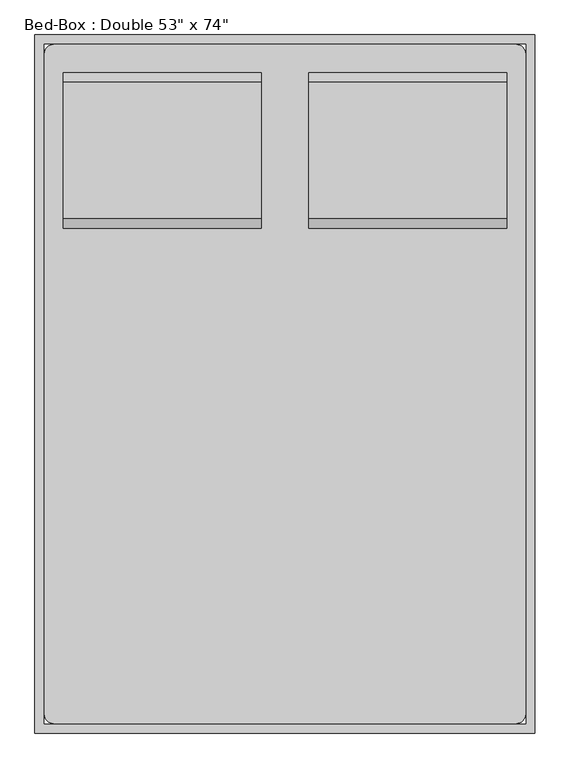
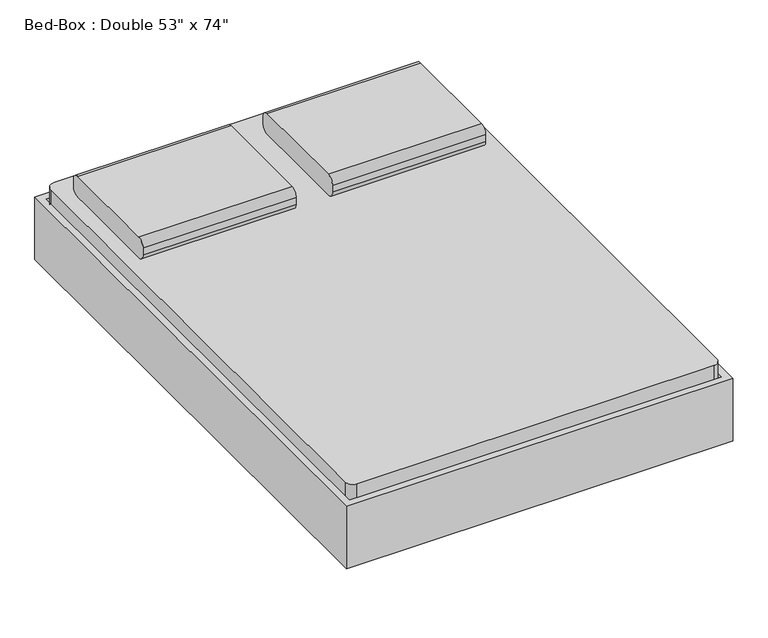
"""IFC4 building model written with IfcOpenShell, lengths in millimetres: furniture geometry."""

from ifc_helpers import new_model, si_unit, point, frame, frame_2d, origin, place, context, project, spatial, polyline, circle_curve, trimmed, segment, composite_curve, outline, extrude, source, transform, mapped, element, save
from ifc_brep_helpers import plane_surface, cylinder_surface, revolved_surface, advanced_brep


def furniture_c8abb964(model_context):
    return source(origin(), model_context, "Body", "SolidModel", [
        extrude(outline(composite_curve([segment(polyline([(578.3704918, 406.4), (210.0704918, 406.4)]), True, "CONTINUOUS"), segment(trimmed(circle_curve(frame_2d((210.0704918, 431.8)), 25.4), [point((210.0704918, 406.4))], [point((184.6704918, 431.8))], False, "CARTESIAN"), True, "CONTINUOUS"), segment(polyline([(184.6704918, 431.8), (184.6704918, 457.2)]), True, "CONTINUOUS"), segment(trimmed(circle_curve(frame_2d((210.0704918, 457.2)), 25.4), [point((184.6704918, 457.2))], [point((210.0704918, 482.6))], False, "CARTESIAN"), True, "CONTINUOUS"), segment(polyline([(210.0704918, 482.6), (578.3704918, 482.6)]), True, "CONTINUOUS"), segment(trimmed(circle_curve(frame_2d((578.3704918, 457.2)), 25.4), [point((578.3704918, 482.6))], [point((603.7704918, 457.2))], False, "CARTESIAN"), True, "CONTINUOUS"), segment(polyline([(603.7704918, 457.2), (603.7704918, 431.8)]), True, "CONTINUOUS"), segment(trimmed(circle_curve(frame_2d((578.3704918, 431.8)), 25.4), [point((603.7704918, 431.8))], [point((578.3704918, 406.4))], False, "CARTESIAN"), True, "CONTINUOUS")], self_intersect=False)), frame((402.652459, 0.0, 0.0), z_axis=(1.0, 0.0, 0.0), x_axis=(0.0, 1.0, 0.0)), (0.0, 0.0, 1.0), 533.4),
        extrude(outline(composite_curve([segment(polyline([(578.3704918, 406.4), (210.0704918, 406.4)]), True, "CONTINUOUS"), segment(trimmed(circle_curve(frame_2d((210.0704918, 431.8)), 25.4), [point((210.0704918, 406.4))], [point((184.6704918, 431.8))], False, "CARTESIAN"), True, "CONTINUOUS"), segment(polyline([(184.6704918, 431.8), (184.6704918, 457.2)]), True, "CONTINUOUS"), segment(trimmed(circle_curve(frame_2d((210.0704918, 457.2)), 25.4), [point((184.6704918, 457.2))], [point((210.0704918, 482.6))], False, "CARTESIAN"), True, "CONTINUOUS"), segment(polyline([(210.0704918, 482.6), (578.3704918, 482.6)]), True, "CONTINUOUS"), segment(trimmed(circle_curve(frame_2d((578.3704918, 457.2)), 25.4), [point((578.3704918, 482.6))], [point((603.7704918, 457.2))], False, "CARTESIAN"), True, "CONTINUOUS"), segment(polyline([(603.7704918, 457.2), (603.7704918, 431.8)]), True, "CONTINUOUS"), segment(trimmed(circle_curve(frame_2d((578.3704918, 431.8)), 25.4), [point((603.7704918, 431.8))], [point((578.3704918, 406.4))], False, "CARTESIAN"), True, "CONTINUOUS")], self_intersect=False)), frame((-257.747541, 0.0, 0.0), z_axis=(1.0, 0.0, 0.0), x_axis=(0.0, 1.0, 0.0)), (0.0, 0.0, 1.0), 533.4),
        advanced_brep(
        [(-308.2231784, 451.3704918, 177.8), (-308.2231784, 375.1704918, 177.8), (-308.2231784, 375.1704918, 196.85), (-308.2231784, 451.3704918, 196.85), (-257.4231784, 451.3704918, 177.8), (-257.4231784, 375.1704918, 177.8), (-245.2869899, 375.1704918, 196.85), (-245.2869899, 451.3704918, 196.85), (-181.3523099, 451.3704918, 14.6654962), (-181.3523099, 375.1704918, 14.6654962), (-164.0871466, 375.1704918, 22.716374), (-164.0871466, 451.3704918, 22.716374), (-158.3320921, 375.1704918, 0.0), (-158.3320921, 451.3704918, 0.0), (-158.3320921, 375.1704918, 19.05), (-158.3320921, 451.3704918, 19.05), (-79.7195862, 451.3704918, 0.0), (-79.7195862, 375.1704918, 0.0), (-79.7195862, 375.1704918, 19.05), (-79.7195862, 451.3704918, 19.05), (-67.0195862, 375.1704918, 3.4029547), (-67.0195862, 451.3704918, 3.4029547), (-76.5445862, 375.1704918, 19.9007387), (-76.5445862, 451.3704918, 19.9007387), (-6.922541, 451.3704918, 38.1), (-6.922541, 375.1704918, 38.1), (-12.0269731, 375.1704918, 57.15), (-12.0269731, 451.3704918, 57.15), (685.5518216, 451.3704918, 38.1), (685.5518216, 375.1704918, 38.1), (690.6562537, 375.1704918, 57.15), (690.6562537, 451.3704918, 57.15), (745.6488669, 451.3704918, 3.4029547), (745.6488669, 375.1704918, 3.4029547), (755.1738669, 375.1704918, 19.9007387), (755.1738669, 451.3704918, 19.9007387), (758.3488669, 375.1704918, 0.0), (758.3488669, 451.3704918, 0.0), (758.3488669, 375.1704918, 19.05), (758.3488669, 451.3704918, 19.05), (836.9613728, 451.3704918, 0.0), (836.9613728, 375.1704918, 0.0), (836.9613728, 375.1704918, 19.05), (836.9613728, 451.3704918, 19.05), (859.9815906, 375.1704918, 14.6654962), (859.9815906, 451.3704918, 14.6654962), (842.7164272, 375.1704918, 22.716374), (842.7164272, 451.3704918, 22.716374), (936.052459, 451.3704918, 177.8), (936.052459, 375.1704918, 177.8), (923.9162705, 375.1704918, 196.85), (923.9162705, 451.3704918, 196.85), (986.852459, 451.3704918, 177.8), (986.852459, 451.3704918, 196.85), (986.852459, 375.1704918, 196.85), (986.852459, 375.1704918, 177.8)],
        [
            (0, 1),
            (1, 2),
            (2, 3),
            (3, 0),
            (0, 4),
            (4, 5),
            (5, 1),
            (5, 6),
            (6, 2),
            (6, 7),
            (7, 3),
            (7, 4),
            (4, 8),
            (8, 9),
            (9, 5),
            (9, 10),
            (10, 6),
            (10, 11),
            (11, 7),
            (11, 8),
            (12, 9, circle_curve(frame((-158.3320921, 375.1704918, 25.4), z_axis=(0.0, 1.0, 0.0), x_axis=(-0.9063077870366486, 0.0, -0.42261826174070233)), 25.4)),
            (8, 13, circle_curve(frame((-158.3320921, 451.3704918, 25.4), z_axis=(0.0, -1.0, 0.0), x_axis=(-0.9063077870366486, 0.0, -0.42261826174070233)), 25.4)),
            (13, 12),
            (14, 10, circle_curve(frame((-158.3320921, 375.1704918, 25.4), z_axis=(0.0, 1.0, 0.0), x_axis=(-0.9063077870366486, 0.0, -0.42261826174070233)), 6.35)),
            (12, 14),
            (15, 11, circle_curve(frame((-158.3320921, 451.3704918, 25.4), z_axis=(0.0, 1.0, 0.0), x_axis=(-0.9063077870366486, 0.0, -0.42261826174070233)), 6.35)),
            (14, 15),
            (15, 13),
            (13, 16),
            (16, 17),
            (17, 12),
            (17, 18),
            (18, 14),
            (18, 19),
            (19, 15),
            (19, 16),
            (20, 17, circle_curve(frame((-79.7195862, 375.1704918, 25.4), z_axis=(0.0, 1.0, 0.0), x_axis=(0.0, 0.0, -1.0)), 25.4)),
            (16, 21, circle_curve(frame((-79.7195862, 451.3704918, 25.4), z_axis=(0.0, -1.0, 0.0), x_axis=(0.0, 0.0, -1.0)), 25.4)),
            (21, 20),
            (22, 18, circle_curve(frame((-79.7195862, 375.1704918, 25.4), z_axis=(0.0, 1.0, 0.0), x_axis=(0.0, 0.0, -1.0)), 6.35)),
            (20, 22),
            (23, 19, circle_curve(frame((-79.7195862, 451.3704918, 25.4), z_axis=(0.0, 1.0, 0.0), x_axis=(0.0, 0.0, -1.0)), 6.35)),
            (22, 23),
            (23, 21),
            (21, 24),
            (24, 25),
            (25, 20),
            (25, 26),
            (26, 22),
            (26, 27),
            (27, 23),
            (27, 24),
            (24, 28),
            (28, 29),
            (29, 25),
            (29, 30),
            (30, 26),
            (30, 31),
            (31, 27),
            (31, 28),
            (28, 32),
            (32, 33),
            (33, 29),
            (33, 34),
            (34, 30),
            (34, 35),
            (35, 31),
            (35, 32),
            (36, 33, circle_curve(frame((758.3488669, 375.1704918, 25.4), z_axis=(0.0, 1.0, 0.0), x_axis=(-0.5000000000000463, 0.0, -0.8660254037844118)), 25.4)),
            (32, 37, circle_curve(frame((758.3488669, 451.3704918, 25.4), z_axis=(0.0, -1.0, 0.0), x_axis=(-0.5000000000000463, 0.0, -0.8660254037844118)), 25.4)),
            (37, 36),
            (38, 34, circle_curve(frame((758.3488669, 375.1704918, 25.4), z_axis=(0.0, 1.0, 0.0), x_axis=(-0.5000000000000463, 0.0, -0.8660254037844118)), 6.35)),
            (36, 38),
            (39, 35, circle_curve(frame((758.3488669, 451.3704918, 25.4), z_axis=(0.0, 1.0, 0.0), x_axis=(-0.5000000000000463, 0.0, -0.8660254037844118)), 6.35)),
            (38, 39),
            (39, 37),
            (37, 40),
            (40, 41),
            (41, 36),
            (41, 42),
            (42, 38),
            (42, 43),
            (43, 39),
            (43, 40),
            (44, 41, circle_curve(frame((836.9613728, 375.1704918, 25.4), z_axis=(0.0, 1.0, 0.0), x_axis=(0.0, 0.0, -1.0)), 25.4)),
            (40, 45, circle_curve(frame((836.9613728, 451.3704918, 25.4), z_axis=(0.0, -1.0, 0.0), x_axis=(0.0, 0.0, -1.0)), 25.4)),
            (45, 44),
            (46, 42, circle_curve(frame((836.9613728, 375.1704918, 25.4), z_axis=(0.0, 1.0, 0.0), x_axis=(0.0, 0.0, -1.0)), 6.35)),
            (44, 46),
            (47, 43, circle_curve(frame((836.9613728, 451.3704918, 25.4), z_axis=(0.0, 1.0, 0.0), x_axis=(0.0, 0.0, -1.0)), 6.35)),
            (46, 47),
            (47, 45),
            (45, 48),
            (48, 49),
            (49, 44),
            (49, 50),
            (50, 46),
            (50, 51),
            (51, 47),
            (51, 48),
            (52, 53),
            (53, 54),
            (54, 55),
            (55, 52),
            (48, 52),
            (55, 49),
            (54, 50),
            (53, 51),
        ],
        [
            plane_surface(frame((-308.2231784, 705.3704918, -152.9490627), z_axis=(-1.0, 0.0, 0.0), x_axis=(0.0, 1.0, 0.0))),
            plane_surface(frame((-308.2231784, 451.3704918, 177.8), z_axis=(0.0, 0.0, -1.0), x_axis=(1.0, 0.0, 0.0))),
            plane_surface(frame((-308.2231784, 375.1704918, 177.8), z_axis=(0.0, -1.0, 0.0), x_axis=(1.0, 0.0, 0.0))),
            plane_surface(frame((-308.2231784, 375.1704918, 196.85), z_axis=(0.0, 0.0, 1.0), x_axis=(1.0, 0.0, 0.0))),
            plane_surface(frame((-308.2231784, 451.3704918, 196.85), z_axis=(0.0, 1.0, 0.0), x_axis=(1.0, 0.0, 0.0))),
            plane_surface(frame((-257.4231784, 451.3704918, 177.8), z_axis=(-0.9063077870366488, 0.0, -0.42261826174070194), x_axis=(0.42261826174070194, 0.0, -0.9063077870366488))),
            plane_surface(frame((-257.4231784, 375.1704918, 177.8), z_axis=(0.0, -1.0, 0.0), x_axis=(0.42261826174070194, 0.0, -0.9063077870366488))),
            plane_surface(frame((-245.2869899, 375.1704918, 196.85), z_axis=(0.9063077870366487, 0.0, 0.4226182617407021), x_axis=(0.4226182617407021, 0.0, -0.9063077870366487))),
            plane_surface(frame((-245.2869899, 451.3704918, 196.85), z_axis=(0.0, 1.0, 0.0), x_axis=(0.4226182617407021, 0.0, -0.9063077870366487))),
            cylinder_surface(frame((-158.3320921, 705.3704918, 25.4), z_axis=(0.0, -1.0, 0.0), x_axis=(-0.9063077870366486, 0.0, -0.42261826174070233)), 25.4),
            plane_surface(frame((-158.3320921, 375.1704918, 25.4), z_axis=(0.0, -1.0, 0.0), x_axis=(-0.9063077870366486, 0.0, -0.42261826174070233))),
            revolved_surface(polyline([(-164.08714654768272, 375.1704918, 22.71637403794654), (-164.08714654768272, 451.3704918, 22.71637403794654)]), (-158.3320921, 705.3704918, 25.4), (0.0, -1.0, 0.0)),
            plane_surface(frame((-158.3320921, 451.3704918, 25.4), z_axis=(0.0, 1.0, 0.0), x_axis=(-0.9063077870366486, 0.0, -0.42261826174070233))),
            plane_surface(frame((-158.3320921, 451.3704918, 0.0), z_axis=(0.0, 0.0, -1.0), x_axis=(1.0, 0.0, 0.0))),
            plane_surface(frame((-158.3320921, 375.1704918, 0.0), z_axis=(0.0, -1.0, 0.0), x_axis=(1.0, 0.0, 0.0))),
            plane_surface(frame((-158.3320921, 375.1704918, 19.05), z_axis=(0.0, 0.0, 1.0), x_axis=(1.0, 0.0, 0.0))),
            plane_surface(frame((-158.3320921, 451.3704918, 19.05), z_axis=(0.0, 1.0, 0.0), x_axis=(1.0, 0.0, 0.0))),
            cylinder_surface(frame((-79.7195862, 705.3704918, 25.4), z_axis=(0.0, -1.0, 0.0), x_axis=(0.0, 0.0, -1.0)), 25.4),
            plane_surface(frame((-79.7195862, 375.1704918, 25.4), z_axis=(0.0, -1.0, 0.0), x_axis=(0.0, 0.0, -1.0))),
            revolved_surface(polyline([(-79.7195862, 375.1704918, 19.049999999999997), (-79.7195862, 451.3704918, 19.049999999999997)]), (-79.7195862, 705.3704918, 25.4), (0.0, -1.0, 0.0)),
            plane_surface(frame((-79.7195862, 451.3704918, 25.4), z_axis=(0.0, 1.0, 0.0), x_axis=(0.0, 0.0, -1.0))),
            plane_surface(frame((-67.0195862, 451.3704918, 3.4029547), z_axis=(0.4999999999998775, 0.0, -0.8660254037845094), x_axis=(0.8660254037845094, 0.0, 0.4999999999998775))),
            plane_surface(frame((-67.0195862, 375.1704918, 3.4029547), z_axis=(0.0, -1.0, 0.0), x_axis=(0.866025403784509, 0.0, 0.49999999999987826))),
            plane_surface(frame((-76.5445862, 375.1704918, 19.9007387), z_axis=(-0.49999999999987754, 0.0, 0.8660254037845093), x_axis=(0.8660254037845093, 0.0, 0.49999999999987754))),
            plane_surface(frame((-76.5445862, 451.3704918, 19.9007387), z_axis=(0.0, 1.0000000000000002, 0.0), x_axis=(0.8660254037845091, 0.0, 0.49999999999987815))),
            plane_surface(frame((-6.922541, 451.3704918, 38.1), z_axis=(0.0, 0.0, -1.0), x_axis=(1.0, 0.0, 0.0))),
            plane_surface(frame((-6.922541, 375.1704918, 38.1), z_axis=(0.0, -1.0, 0.0), x_axis=(1.0, 0.0, 0.0))),
            plane_surface(frame((-12.0269731, 375.1704918, 57.15), z_axis=(0.0, 0.0, 1.0), x_axis=(1.0, 0.0, 0.0))),
            plane_surface(frame((-12.0269731, 451.3704918, 57.15), z_axis=(0.0, 1.0, 0.0), x_axis=(1.0, 0.0, 0.0))),
            plane_surface(frame((685.5518216, 451.3704918, 38.1), z_axis=(-0.500000000000047, 0.0, -0.8660254037844116), x_axis=(0.8660254037844116, 0.0, -0.500000000000047))),
            plane_surface(frame((685.5518216, 375.1704918, 38.1), z_axis=(0.0, -1.0, 0.0), x_axis=(0.8660254037844122, 0.0, -0.5000000000000459))),
            plane_surface(frame((690.6562537, 375.1704918, 57.15), z_axis=(0.5000000000000461, 0.0, 0.8660254037844121), x_axis=(0.8660254037844121, 0.0, -0.5000000000000461))),
            plane_surface(frame((690.6562537, 451.3704918, 57.15), z_axis=(0.0, 1.0, 0.0), x_axis=(0.8660254037844127, 0.0, -0.500000000000045))),
            cylinder_surface(frame((758.3488669, 705.3704918, 25.4), z_axis=(0.0, -1.0, 0.0), x_axis=(-0.5000000000000463, 0.0, -0.8660254037844118)), 25.4),
            plane_surface(frame((758.3488669, 375.1704918, 25.4), z_axis=(0.0, -1.0000000000000002, 0.0), x_axis=(-0.5000000000000464, 0.0, -0.866025403784412))),
            revolved_surface(polyline([(755.1738668999997, 375.1704918, 19.90073868596898), (755.1738668999997, 451.3704918, 19.90073868596898)]), (758.3488669, 705.3704918, 25.4), (0.0, -1.0, 0.0)),
            plane_surface(frame((758.3488669, 451.3704918, 25.4), z_axis=(0.0, 1.0000000000000002, 0.0), x_axis=(-0.5000000000000464, 0.0, -0.866025403784412))),
            plane_surface(frame((758.3488669, 451.3704918, 0.0), z_axis=(0.0, 0.0, -1.0), x_axis=(1.0, 0.0, 0.0))),
            plane_surface(frame((758.3488669, 375.1704918, 0.0), z_axis=(0.0, -1.0, 0.0), x_axis=(1.0, 0.0, 0.0))),
            plane_surface(frame((758.3488669, 375.1704918, 19.05), z_axis=(0.0, 0.0, 1.0), x_axis=(1.0, 0.0, 0.0))),
            plane_surface(frame((758.3488669, 451.3704918, 19.05), z_axis=(0.0, 1.0, 0.0), x_axis=(1.0, 0.0, 0.0))),
            cylinder_surface(frame((836.9613728, 705.3704918, 25.4), z_axis=(0.0, -1.0, 0.0), x_axis=(0.0, 0.0, -1.0)), 25.4),
            plane_surface(frame((836.9613728, 375.1704918, 25.4), z_axis=(0.0, -1.0, 0.0), x_axis=(0.0, 0.0, -1.0))),
            revolved_surface(polyline([(836.9613728, 375.1704918, 19.049999999999997), (836.9613728, 451.3704918, 19.049999999999997)]), (836.9613728, 705.3704918, 25.4), (0.0, -1.0, 0.0)),
            plane_surface(frame((836.9613728, 451.3704918, 25.4), z_axis=(0.0, 1.0, 0.0), x_axis=(0.0, 0.0, -1.0))),
            plane_surface(frame((859.9815906, 451.3704918, 14.6654962), z_axis=(0.9063077870366797, 0.0, -0.42261826174063566), x_axis=(0.42261826174063566, 0.0, 0.9063077870366797))),
            plane_surface(frame((859.9815906, 375.1704918, 14.6654962), z_axis=(0.0, -1.0000000000000002, 0.0), x_axis=(0.4226182617406349, 0.0, 0.9063077870366801))),
            plane_surface(frame((842.7164272, 375.1704918, 22.716374), z_axis=(-0.9063077870366799, 0.0, 0.4226182617406354), x_axis=(0.4226182617406354, 0.0, 0.9063077870366799))),
            plane_surface(frame((842.7164272, 451.3704918, 22.716374), z_axis=(0.0, 1.0, 0.0), x_axis=(0.42261826174063555, 0.0, 0.9063077870366798))),
            plane_surface(frame((986.852459, 705.3704918, -152.9490627), z_axis=(1.0, 0.0, 0.0), x_axis=(0.0, 1.0, 0.0))),
            plane_surface(frame((936.052459, 451.3704918, 177.8), z_axis=(0.0, 0.0, -1.0), x_axis=(1.0, 0.0, 0.0))),
            plane_surface(frame((936.052459, 375.1704918, 177.8), z_axis=(0.0, -1.0, 0.0), x_axis=(1.0, 0.0, 0.0))),
            plane_surface(frame((923.9162705, 375.1704918, 196.85), z_axis=(0.0, 0.0, 1.0), x_axis=(1.0, 0.0, 0.0))),
            plane_surface(frame((923.9162705, 451.3704918, 196.85), z_axis=(0.0, 1.0, 0.0), x_axis=(1.0, 0.0, 0.0))),
        ],
        [
            (0, [[1, 2, 3, 4]]),
            (1, [[-1, 5, 6, 7]]),
            (2, [[-2, -7, 8, 9]]),
            (3, [[-3, -9, 10, 11]]),
            (4, [[-4, -11, 12, -5]]),
            (5, [[-6, 13, 14, 15]]),
            (6, [[-8, -15, 16, 17]]),
            (7, [[-10, -17, 18, 19]]),
            (8, [[-12, -19, 20, -13]]),
            (9, [[21, -14, 22, 23]]),
            (10, [[24, -16, -21, 25]]),
            (11, [[26, -18, -24, 27]]),
            (12, [[-22, -20, -26, 28]]),
            (13, [[-23, 29, 30, 31]]),
            (14, [[-25, -31, 32, 33]]),
            (15, [[-27, -33, 34, 35]]),
            (16, [[-28, -35, 36, -29]]),
            (17, [[37, -30, 38, 39]]),
            (18, [[40, -32, -37, 41]]),
            (19, [[42, -34, -40, 43]]),
            (20, [[-38, -36, -42, 44]]),
            (21, [[-39, 45, 46, 47]]),
            (22, [[-41, -47, 48, 49]]),
            (23, [[-43, -49, 50, 51]]),
            (24, [[-44, -51, 52, -45]]),
            (25, [[-46, 53, 54, 55]]),
            (26, [[-48, -55, 56, 57]]),
            (27, [[-50, -57, 58, 59]]),
            (28, [[-52, -59, 60, -53]]),
            (29, [[-54, 61, 62, 63]]),
            (30, [[-56, -63, 64, 65]]),
            (31, [[-58, -65, 66, 67]]),
            (32, [[-60, -67, 68, -61]]),
            (33, [[69, -62, 70, 71]]),
            (34, [[72, -64, -69, 73]]),
            (35, [[74, -66, -72, 75]]),
            (36, [[-70, -68, -74, 76]]),
            (37, [[-71, 77, 78, 79]]),
            (38, [[-73, -79, 80, 81]]),
            (39, [[-75, -81, 82, 83]]),
            (40, [[-76, -83, 84, -77]]),
            (41, [[85, -78, 86, 87]]),
            (42, [[88, -80, -85, 89]]),
            (43, [[90, -82, -88, 91]]),
            (44, [[-86, -84, -90, 92]]),
            (45, [[-87, 93, 94, 95]]),
            (46, [[-89, -95, 96, 97]]),
            (47, [[-91, -97, 98, 99]]),
            (48, [[-92, -99, 100, -93]]),
            (49, [[101, 102, 103, 104]]),
            (50, [[-94, 105, -104, 106]]),
            (51, [[-96, -106, -103, 107]]),
            (52, [[-98, -107, -102, 108]]),
            (53, [[-100, -108, -101, -105]]),
        ],
    ),
        extrude(outline(composite_curve([segment(polyline([(-283.147541, 679.9704918), (961.452459, 679.9704918)]), True, "CONTINUOUS"), segment(trimmed(circle_curve(frame_2d((961.452459, 654.5704918)), 25.4), [point((961.452459, 679.9704918))], [point((986.852459, 654.5704918))], False, "CARTESIAN"), True, "CONTINUOUS"), segment(polyline([(986.852459, 654.5704918), (986.852459, -1123.4295082)]), True, "CONTINUOUS"), segment(trimmed(circle_curve(frame_2d((961.452459, -1123.4295082)), 25.4), [point((986.852459, -1123.4295082))], [point((961.452459, -1148.8295082))], False, "CARTESIAN"), True, "CONTINUOUS"), segment(polyline([(961.452459, -1148.8295082), (-283.147541, -1148.8295082)]), True, "CONTINUOUS"), segment(trimmed(circle_curve(frame_2d((-283.147541, -1123.4295082)), 25.4), [point((-283.147541, -1148.8295082))], [point((-308.547541, -1123.4295082))], False, "CARTESIAN"), True, "CONTINUOUS"), segment(polyline([(-308.547541, -1123.4295082), (-308.547541, 654.5704918)]), True, "CONTINUOUS"), segment(trimmed(circle_curve(frame_2d((-283.147541, 654.5704918)), 25.4), [point((-308.547541, 654.5704918))], [point((-283.147541, 679.9704918))], False, "CARTESIAN"), True, "CONTINUOUS")], self_intersect=False)), frame((0.0, 0.0, 203.2), z_axis=(0.0, 0.0, 1.0), x_axis=(1.0, 0.0, 0.0)), (0.0, 0.0, 1.0), 203.2),
        advanced_brep(
        [(-308.547541, -869.4295082, 196.85), (-308.547541, -869.4295082, 177.8), (-308.547541, -945.6295082, 177.8), (-308.547541, -945.6295082, 196.85), (-245.6113525, -869.4295082, 196.85), (-257.747541, -869.4295082, 177.8), (-257.747541, -945.6295082, 177.8), (-245.6113525, -945.6295082, 196.85), (-164.4115092, -869.4295082, 22.716374), (-181.6766725, -869.4295082, 14.6654962), (-181.6766725, -945.6295082, 14.6654962), (-164.4115092, -945.6295082, 22.716374), (-158.6564547, -869.4295082, 0.0), (-158.6564547, -869.4295082, 19.05), (-158.6564547, -945.6295082, 0.0), (-158.6564547, -945.6295082, 19.05), (-80.0439489, -869.4295082, 19.05), (-80.0439489, -869.4295082, 0.0), (-80.0439489, -945.6295082, 0.0), (-80.0439489, -945.6295082, 19.05), (-67.3439489, -869.4295082, 3.4029547), (-76.8689489, -869.4295082, 19.9007387), (-67.3439489, -945.6295082, 3.4029547), (-76.8689489, -945.6295082, 19.9007387), (-12.3513357, -869.4295082, 57.15), (-7.2469036, -869.4295082, 38.1), (-7.2469036, -945.6295082, 38.1), (-12.3513357, -945.6295082, 57.15), (690.6562537, -869.4295082, 57.15), (685.5518216, -869.4295082, 38.1), (685.5518216, -945.6295082, 38.1), (690.6562537, -945.6295082, 57.15), (755.1738669, -869.4295082, 19.9007387), (745.6488669, -869.4295082, 3.4029547), (745.6488669, -945.6295082, 3.4029547), (755.1738669, -945.6295082, 19.9007387), (758.3488669, -869.4295082, 0.0), (758.3488669, -869.4295082, 19.05), (758.3488669, -945.6295082, 0.0), (758.3488669, -945.6295082, 19.05), (836.9613728, -869.4295082, 19.05), (836.9613728, -869.4295082, 0.0), (836.9613728, -945.6295082, 0.0), (836.9613728, -945.6295082, 19.05), (859.9815906, -869.4295082, 14.6654962), (842.7164272, -869.4295082, 22.716374), (859.9815906, -945.6295082, 14.6654962), (842.7164272, -945.6295082, 22.716374), (923.9162705, -869.4295082, 196.85), (936.052459, -869.4295082, 177.8), (936.052459, -945.6295082, 177.8), (923.9162705, -945.6295082, 196.85), (986.852459, -869.4295082, 196.85), (986.852459, -945.6295082, 196.85), (986.852459, -945.6295082, 177.8), (986.852459, -869.4295082, 177.8)],
        [
            (0, 1),
            (1, 2),
            (2, 3),
            (3, 0),
            (0, 4),
            (4, 5),
            (5, 1),
            (5, 6),
            (6, 2),
            (6, 7),
            (7, 3),
            (7, 4),
            (4, 8),
            (8, 9),
            (9, 5),
            (9, 10),
            (10, 6),
            (10, 11),
            (11, 7),
            (11, 8),
            (12, 9, circle_curve(frame((-158.6564547, -869.4295082, 25.4), z_axis=(0.0, 1.0, 0.0), x_axis=(-0.906307787036663, 0.0, -0.4226182617406713)), 25.4)),
            (8, 13, circle_curve(frame((-158.6564547, -869.4295082, 25.4), z_axis=(0.0, -1.0, 0.0), x_axis=(-0.906307787036663, 0.0, -0.4226182617406713)), 6.35)),
            (13, 12),
            (14, 10, circle_curve(frame((-158.6564547, -945.6295082, 25.4), z_axis=(0.0, 1.0, 0.0), x_axis=(-0.906307787036663, 0.0, -0.4226182617406713)), 25.4)),
            (12, 14),
            (15, 11, circle_curve(frame((-158.6564547, -945.6295082, 25.4), z_axis=(0.0, 1.0, 0.0), x_axis=(-0.906307787036663, 0.0, -0.4226182617406713)), 6.35)),
            (14, 15),
            (15, 13),
            (13, 16),
            (16, 17),
            (17, 12),
            (17, 18),
            (18, 14),
            (18, 19),
            (19, 15),
            (19, 16),
            (20, 17, circle_curve(frame((-80.0439489, -869.4295082, 25.4), z_axis=(0.0, 1.0, 0.0), x_axis=(0.0, 0.0, -1.0)), 25.4)),
            (16, 21, circle_curve(frame((-80.0439489, -869.4295082, 25.4), z_axis=(0.0, -1.0, 0.0), x_axis=(0.0, 0.0, -1.0)), 6.35)),
            (21, 20),
            (22, 18, circle_curve(frame((-80.0439489, -945.6295082, 25.4), z_axis=(0.0, 1.0, 0.0), x_axis=(0.0, 0.0, -1.0)), 25.4)),
            (20, 22),
            (23, 19, circle_curve(frame((-80.0439489, -945.6295082, 25.4), z_axis=(0.0, 1.0, 0.0), x_axis=(0.0, 0.0, -1.0)), 6.35)),
            (22, 23),
            (23, 21),
            (21, 24),
            (24, 25),
            (25, 20),
            (25, 26),
            (26, 22),
            (26, 27),
            (27, 23),
            (27, 24),
            (24, 28),
            (28, 29),
            (29, 25),
            (29, 30),
            (30, 26),
            (30, 31),
            (31, 27),
            (31, 28),
            (28, 32),
            (32, 33),
            (33, 29),
            (33, 34),
            (34, 30),
            (34, 35),
            (35, 31),
            (35, 32),
            (36, 33, circle_curve(frame((758.3488669, -869.4295082, 25.4), z_axis=(0.0, 1.0, 0.0), x_axis=(-0.5000000000000479, 0.0, -0.866025403784411)), 25.4)),
            (32, 37, circle_curve(frame((758.3488669, -869.4295082, 25.4), z_axis=(0.0, -1.0, 0.0), x_axis=(-0.5000000000000479, 0.0, -0.866025403784411)), 6.35)),
            (37, 36),
            (38, 34, circle_curve(frame((758.3488669, -945.6295082, 25.4), z_axis=(0.0, 1.0, 0.0), x_axis=(-0.5000000000000479, 0.0, -0.866025403784411)), 25.4)),
            (36, 38),
            (39, 35, circle_curve(frame((758.3488669, -945.6295082, 25.4), z_axis=(0.0, 1.0, 0.0), x_axis=(-0.5000000000000479, 0.0, -0.866025403784411)), 6.35)),
            (38, 39),
            (39, 37),
            (37, 40),
            (40, 41),
            (41, 36),
            (41, 42),
            (42, 38),
            (42, 43),
            (43, 39),
            (43, 40),
            (44, 41, circle_curve(frame((836.9613728, -869.4295082, 25.4), z_axis=(0.0, 1.0, 0.0), x_axis=(0.0, 0.0, -1.0)), 25.4)),
            (40, 45, circle_curve(frame((836.9613728, -869.4295082, 25.4), z_axis=(0.0, -1.0, 0.0), x_axis=(0.0, 0.0, -1.0)), 6.35)),
            (45, 44),
            (46, 42, circle_curve(frame((836.9613728, -945.6295082, 25.4), z_axis=(0.0, 1.0, 0.0), x_axis=(0.0, 0.0, -1.0)), 25.4)),
            (44, 46),
            (47, 43, circle_curve(frame((836.9613728, -945.6295082, 25.4), z_axis=(0.0, 1.0, 0.0), x_axis=(0.0, 0.0, -1.0)), 6.35)),
            (46, 47),
            (47, 45),
            (45, 48),
            (48, 49),
            (49, 44),
            (49, 50),
            (50, 46),
            (50, 51),
            (51, 47),
            (51, 48),
            (52, 53),
            (53, 54),
            (54, 55),
            (55, 52),
            (48, 52),
            (55, 49),
            (54, 50),
            (53, 51),
        ],
        [
            plane_surface(frame((-308.547541, -1174.2295082, -127.5947323), z_axis=(-1.0, 0.0, 0.0), x_axis=(0.0, 1.0, 0.0))),
            plane_surface(frame((-308.547541, -869.4295082, 196.85), z_axis=(0.0, 1.0, 0.0), x_axis=(1.0, 0.0, 0.0))),
            plane_surface(frame((-308.547541, -869.4295082, 177.8), z_axis=(0.0, 0.0, -1.0), x_axis=(1.0, 0.0, 0.0))),
            plane_surface(frame((-308.547541, -945.6295082, 177.8), z_axis=(0.0, -1.0, 0.0), x_axis=(1.0, 0.0, 0.0))),
            plane_surface(frame((-308.547541, -945.6295082, 196.85), z_axis=(0.0, 0.0, 1.0), x_axis=(1.0, 0.0, 0.0))),
            plane_surface(frame((-245.6113525, -869.4295082, 196.85), z_axis=(0.0, 1.0, 0.0), x_axis=(0.422618261740671, 0.0, -0.9063077870366633))),
            plane_surface(frame((-257.747541, -869.4295082, 177.8), z_axis=(-0.9063077870366631, 0.0, -0.42261826174067113), x_axis=(0.42261826174067113, 0.0, -0.9063077870366631))),
            plane_surface(frame((-257.747541, -945.6295082, 177.8), z_axis=(0.0, -1.0, 0.0), x_axis=(0.42261826174067135, 0.0, -0.906307787036663))),
            plane_surface(frame((-245.6113525, -945.6295082, 196.85), z_axis=(0.9063077870366631, 0.0, 0.4226182617406713), x_axis=(0.4226182617406713, 0.0, -0.9063077870366631))),
            plane_surface(frame((-158.6564547, -869.4295082, 25.4), z_axis=(0.0, 1.0, 0.0), x_axis=(-0.906307787036663, 0.0, -0.4226182617406713))),
            cylinder_surface(frame((-158.6564547, -1174.2295082, 25.4), z_axis=(0.0, -1.0, 0.0), x_axis=(-0.906307787036663, 0.0, -0.4226182617406713)), 25.4),
            plane_surface(frame((-158.6564547, -945.6295082, 25.4), z_axis=(0.0, -1.0, 0.0), x_axis=(-0.906307787036663, 0.0, -0.4226182617406713))),
            revolved_surface(polyline([(-164.41150914768284, -945.6295082, 22.716374037946736), (-164.41150914768284, -869.4295082, 22.716374037946736)]), (-158.6564547, -1174.2295082, 25.4), (0.0, -1.0, 0.0)),
            plane_surface(frame((-158.6564547, -869.4295082, 19.05), z_axis=(0.0, 1.0, 0.0), x_axis=(1.0, 0.0, 0.0))),
            plane_surface(frame((-158.6564547, -869.4295082, 0.0), z_axis=(0.0, 0.0, -1.0), x_axis=(1.0, 0.0, 0.0))),
            plane_surface(frame((-158.6564547, -945.6295082, 0.0), z_axis=(0.0, -1.0, 0.0), x_axis=(1.0, 0.0, 0.0))),
            plane_surface(frame((-158.6564547, -945.6295082, 19.05), z_axis=(0.0, 0.0, 1.0), x_axis=(1.0, 0.0, 0.0))),
            plane_surface(frame((-80.0439489, -869.4295082, 25.4), z_axis=(0.0, 1.0, 0.0), x_axis=(0.0, 0.0, -1.0))),
            cylinder_surface(frame((-80.0439489, -1174.2295082, 25.4), z_axis=(0.0, -1.0, 0.0), x_axis=(0.0, 0.0, -1.0)), 25.4),
            plane_surface(frame((-80.0439489, -945.6295082, 25.4), z_axis=(0.0, -1.0, 0.0), x_axis=(0.0, 0.0, -1.0))),
            revolved_surface(polyline([(-80.0439489, -945.6295082, 19.049999999999997), (-80.0439489, -869.4295082, 19.049999999999997)]), (-80.0439489, -1174.2295082, 25.4), (0.0, -1.0, 0.0)),
            plane_surface(frame((-76.8689489, -869.4295082, 19.9007387), z_axis=(0.0, 1.0, 0.0), x_axis=(0.8660254037844785, 0.0, 0.499999999999931))),
            plane_surface(frame((-67.3439489, -869.4295082, 3.4029547), z_axis=(0.499999999999931, 0.0, -0.8660254037844785), x_axis=(0.8660254037844785, 0.0, 0.499999999999931))),
            plane_surface(frame((-67.3439489, -945.6295082, 3.4029547), z_axis=(0.0, -1.0, 0.0), x_axis=(0.8660254037844786, 0.0, 0.49999999999993094))),
            plane_surface(frame((-76.8689489, -945.6295082, 19.9007387), z_axis=(-0.4999999999999312, 0.0, 0.8660254037844785), x_axis=(0.8660254037844785, 0.0, 0.4999999999999312))),
            plane_surface(frame((-12.3513357, -869.4295082, 57.15), z_axis=(0.0, 1.0, 0.0), x_axis=(1.0, 0.0, 0.0))),
            plane_surface(frame((-7.2469036, -869.4295082, 38.1), z_axis=(0.0, 0.0, -1.0), x_axis=(1.0, 0.0, 0.0))),
            plane_surface(frame((-7.2469036, -945.6295082, 38.1), z_axis=(0.0, -1.0, 0.0), x_axis=(1.0, 0.0, 0.0))),
            plane_surface(frame((-12.3513357, -945.6295082, 57.15), z_axis=(0.0, 0.0, 1.0), x_axis=(1.0, 0.0, 0.0))),
            plane_surface(frame((690.6562537, -869.4295082, 57.15), z_axis=(0.0, 1.0, 0.0), x_axis=(0.8660254037844091, 0.0, -0.5000000000000514))),
            plane_surface(frame((685.5518216, -869.4295082, 38.1), z_axis=(-0.5000000000000502, 0.0, -0.8660254037844097), x_axis=(0.8660254037844097, 0.0, -0.5000000000000502))),
            plane_surface(frame((685.5518216, -945.6295082, 38.1), z_axis=(0.0, -1.0, 0.0), x_axis=(0.86602540378441, 0.0, -0.5000000000000498))),
            plane_surface(frame((690.6562537, -945.6295082, 57.15), z_axis=(0.5000000000000505, 0.0, 0.8660254037844095), x_axis=(0.8660254037844095, 0.0, -0.5000000000000505))),
            plane_surface(frame((758.3488669, -869.4295082, 25.4), z_axis=(0.0, 1.0000000000000002, 0.0), x_axis=(-0.500000000000048, 0.0, -0.8660254037844111))),
            cylinder_surface(frame((758.3488669, -1174.2295082, 25.4), z_axis=(0.0, -1.0, 0.0), x_axis=(-0.5000000000000479, 0.0, -0.866025403784411)), 25.4),
            plane_surface(frame((758.3488669, -945.6295082, 25.4), z_axis=(0.0, -1.0000000000000002, 0.0), x_axis=(-0.500000000000048, 0.0, -0.8660254037844111))),
            revolved_surface(polyline([(755.1738668999997, -945.6295082, 19.90073868596899), (755.1738668999997, -869.4295082, 19.90073868596899)]), (758.3488669, -1174.2295082, 25.4), (0.0, -1.0, 0.0)),
            plane_surface(frame((758.3488669, -869.4295082, 19.05), z_axis=(0.0, 1.0, 0.0), x_axis=(1.0, 0.0, 0.0))),
            plane_surface(frame((758.3488669, -869.4295082, 0.0), z_axis=(0.0, 0.0, -1.0), x_axis=(1.0, 0.0, 0.0))),
            plane_surface(frame((758.3488669, -945.6295082, 0.0), z_axis=(0.0, -1.0, 0.0), x_axis=(1.0, 0.0, 0.0))),
            plane_surface(frame((758.3488669, -945.6295082, 19.05), z_axis=(0.0, 0.0, 1.0), x_axis=(1.0, 0.0, 0.0))),
            plane_surface(frame((836.9613728, -869.4295082, 25.4), z_axis=(0.0, 1.0, 0.0), x_axis=(0.0, 0.0, -1.0))),
            cylinder_surface(frame((836.9613728, -1174.2295082, 25.4), z_axis=(0.0, -1.0, 0.0), x_axis=(0.0, 0.0, -1.0)), 25.4),
            plane_surface(frame((836.9613728, -945.6295082, 25.4), z_axis=(0.0, -1.0, 0.0), x_axis=(0.0, 0.0, -1.0))),
            revolved_surface(polyline([(836.9613728, -945.6295082, 19.049999999999997), (836.9613728, -869.4295082, 19.049999999999997)]), (836.9613728, -1174.2295082, 25.4), (0.0, -1.0, 0.0)),
            plane_surface(frame((842.7164272, -869.4295082, 22.716374), z_axis=(0.0, 1.0, 0.0), x_axis=(0.4226182617405411, 0.0, 0.9063077870367238))),
            plane_surface(frame((859.9815906, -869.4295082, 14.6654962), z_axis=(0.9063077870367237, 0.0, -0.42261826174054157), x_axis=(0.42261826174054157, 0.0, 0.9063077870367237))),
            plane_surface(frame((859.9815906, -945.6295082, 14.6654962), z_axis=(0.0, -1.0, 0.0), x_axis=(0.4226182617405412, 0.0, 0.9063077870367238))),
            plane_surface(frame((842.7164272, -945.6295082, 22.716374), z_axis=(-0.906307787036724, 0.0, 0.422618261740541), x_axis=(0.422618261740541, 0.0, 0.906307787036724))),
            plane_surface(frame((986.852459, -1174.2295082, -127.5947323), z_axis=(1.0, 0.0, 0.0), x_axis=(0.0, 1.0, 0.0))),
            plane_surface(frame((923.9162705, -869.4295082, 196.85), z_axis=(0.0, 1.0, 0.0), x_axis=(1.0, 0.0, 0.0))),
            plane_surface(frame((936.052459, -869.4295082, 177.8), z_axis=(0.0, 0.0, -1.0), x_axis=(1.0, 0.0, 0.0))),
            plane_surface(frame((936.052459, -945.6295082, 177.8), z_axis=(0.0, -1.0, 0.0), x_axis=(1.0, 0.0, 0.0))),
            plane_surface(frame((923.9162705, -945.6295082, 196.85), z_axis=(0.0, 0.0, 1.0), x_axis=(1.0, 0.0, 0.0))),
        ],
        [
            (0, [[1, 2, 3, 4]]),
            (1, [[-1, 5, 6, 7]]),
            (2, [[-2, -7, 8, 9]]),
            (3, [[-3, -9, 10, 11]]),
            (4, [[-4, -11, 12, -5]]),
            (5, [[-6, 13, 14, 15]]),
            (6, [[-8, -15, 16, 17]]),
            (7, [[-10, -17, 18, 19]]),
            (8, [[-12, -19, 20, -13]]),
            (9, [[21, -14, 22, 23]]),
            (10, [[24, -16, -21, 25]]),
            (11, [[26, -18, -24, 27]]),
            (12, [[-22, -20, -26, 28]]),
            (13, [[-23, 29, 30, 31]]),
            (14, [[-25, -31, 32, 33]]),
            (15, [[-27, -33, 34, 35]]),
            (16, [[-28, -35, 36, -29]]),
            (17, [[37, -30, 38, 39]]),
            (18, [[40, -32, -37, 41]]),
            (19, [[42, -34, -40, 43]]),
            (20, [[-38, -36, -42, 44]]),
            (21, [[-39, 45, 46, 47]]),
            (22, [[-41, -47, 48, 49]]),
            (23, [[-43, -49, 50, 51]]),
            (24, [[-44, -51, 52, -45]]),
            (25, [[-46, 53, 54, 55]]),
            (26, [[-48, -55, 56, 57]]),
            (27, [[-50, -57, 58, 59]]),
            (28, [[-52, -59, 60, -53]]),
            (29, [[-54, 61, 62, 63]]),
            (30, [[-56, -63, 64, 65]]),
            (31, [[-58, -65, 66, 67]]),
            (32, [[-60, -67, 68, -61]]),
            (33, [[69, -62, 70, 71]]),
            (34, [[72, -64, -69, 73]]),
            (35, [[74, -66, -72, 75]]),
            (36, [[-70, -68, -74, 76]]),
            (37, [[-71, 77, 78, 79]]),
            (38, [[-73, -79, 80, 81]]),
            (39, [[-75, -81, 82, 83]]),
            (40, [[-76, -83, 84, -77]]),
            (41, [[85, -78, 86, 87]]),
            (42, [[88, -80, -85, 89]]),
            (43, [[90, -82, -88, 91]]),
            (44, [[-86, -84, -90, 92]]),
            (45, [[-87, 93, 94, 95]]),
            (46, [[-89, -95, 96, 97]]),
            (47, [[-91, -97, 98, 99]]),
            (48, [[-92, -99, 100, -93]]),
            (49, [[101, 102, 103, 104]]),
            (50, [[-94, 105, -104, 106]]),
            (51, [[-96, -106, -103, 107]]),
            (52, [[-98, -107, -102, 108]]),
            (53, [[-100, -108, -101, -105]]),
        ],
    ),
        extrude(outline(polyline([(1012.252459, 705.3704918), (1012.252459, -1174.2295082), (-333.947541, -1174.2295082), (-333.947541, 705.3704918), (1012.252459, 705.3704918)]), holes=[polyline([(986.852459, 679.9704918), (-308.547541, 679.9704918), (-308.547541, -1148.8295082), (986.852459, -1148.8295082), (986.852459, 679.9704918)])]), frame((0.0, 0.0, 127.0), z_axis=(0.0, 0.0, 1.0), x_axis=(1.0, 0.0, 0.0)), (0.0, 0.0, 1.0), 228.6),
    ])


if __name__ == "__main__":
    model = new_model("IFC4")
    model_context = context("Model", 3, world=origin())
    ifc_project = project(units=[si_unit("LENGTHUNIT", "METRE", prefix="MILLI")], contexts=[model_context])
    site = spatial("IfcSite", under=ifc_project)
    building = spatial("IfcBuilding", under=site)
    placement = place(None, origin())
    furniture_shape = furniture_c8abb964(model_context)
    element("IfcFurniture", 1, ObjectType="Bed-Box : Double 53\" x 74\"", at=placement, inside=building, context=model_context, shape_type="MappedRepresentation", body=[
        mapped(furniture_shape, transform((0.0, 0.0, 0.0), x_axis=(1.0, 0.0, 0.0), y_axis=(0.0, 1.0, 0.0), z_axis=(0.0, 0.0, 1.0))),
    ])
    save(model, "model.ifc")

# Revit data of these elements
# Type "Bed-Box : Double 53\" x 74\""
#   Assembly Code = "E2020200"
#   Length = 6' - 2"
#   Width = 4' - 5"
#   Frame Material = Birch
#   Mattress Material = Sash
#   Default Elevation = 0
# Element 1 (IfcFurniture, "Bed-Box : Double 53\" x 74\"")
#   Materials on its faces: "Birch", "Sash"
# Materials
#   "Birch": class "Wood", colour RGB 224 178 126, transparency 0, Description = "Betula Alleghaniensis", Cost = 0
#   "Sash": class "Wood", colour RGB 224 178 126, transparency 0
